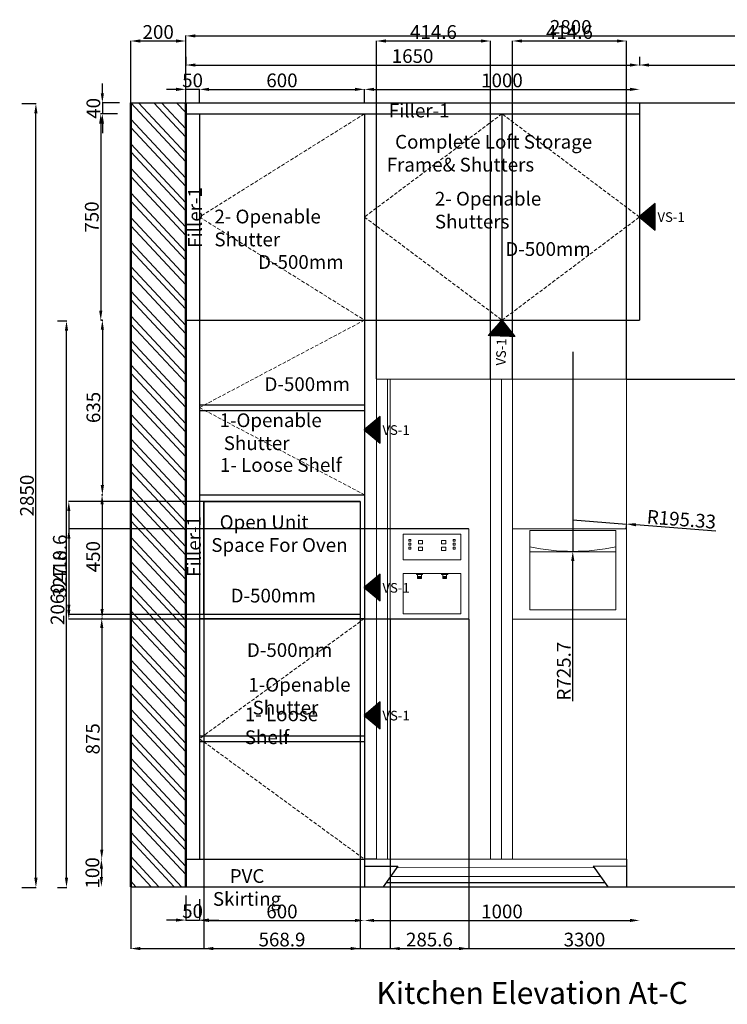
# Model space of a CAD drawing. Units: millimetres. Extents: x 407065 to 421840, y 1168257 to 1177792.
# Tile 1 of 17: x 407430 to 410003, y 1168257 to 1171838. Entities that reach past the tile are written whole.
import ezdxf

# ---------------------------------------------------------------- set-up
doc = ezdxf.new("R2010")
doc.units = ezdxf.units.MM
doc.linetypes.add('DASHED', pattern=[19.05, 12.7, -6.35])
for name, color, linetype, lineweight in [('A-ANNO-DIMS', 6, 'Continuous', 18), ('A-ANNO-TEXT', 30, 'Continuous', 18), ('A-EQPM', 8, 'Continuous', 18), ('A-FURN', 3, 'Continuous', 25), ('A-FURN-HIDN', 7, 'DASHED', 18), ('A-WALL', 7, 'Continuous', 50), ('A-WALL-PATT', 8, 'Continuous', 13)]:
    doc.layers.add(name, color=color, linetype=linetype, lineweight=lineweight)
doc.styles.get("Standard").update_dxf_attribs({"font": 'arial.ttf'})
doc.dimstyles.new('ISO-25', dxfattribs={"dimtxt": 50, "dimasz": 35, "dimexe": 1.25, "dimexo": 0.625, "dimtad": 1, "dimdec": 1, "dimtxsty": 'Standard', "dimcen": 35, "dimadec": 0, "dimazin": 0, "dimtfac": 1, "dimtdec": 1, "dimtmove": 0, "dimatfit": 3, "dimfxl": 1, "dimarcsym": 0})

# ---------------------------------------------------------------- blocks, each defined once
blk = doc.blocks.new('*D118')
at = {"layer": 'A-ANNO-DIMS', "color": 0, "lineweight": -2, "transparency": 16777216}
for p, q in [((407998.5, 1171584.4), (407963.5, 1171584.4)), ((408033.5, 1171554), (408033.5, 1171585.6)), ((408083.5, 1171584.4), (408033.5, 1171584.4)), ((408083.5, 1171541.4), (408083.5, 1171585.6)), ((408118.5, 1171584.4), (408153.5, 1171584.4))]:
    blk.add_line(p, q, dxfattribs=at)
at = {"layer": 'A-ANNO-DIMS', "color": 0, "transparency": 16777216}
for points in [[(407998.5, 1171590.2), (407998.5, 1171578.5), (408033.5, 1171584.4)], [(408118.5, 1171590.2), (408118.5, 1171578.5), (408083.5, 1171584.4)]]:
    blk.add_solid(points, dxfattribs=at)
at = {"layer": 'Defpoints', "color": 0, "transparency": 16777216}
for p in [(408033.5, 1171584.4), (408033.5, 1171553.4), (408083.5, 1171540.7)]:
    blk.add_point(p, dxfattribs=at)
at = {"layer": 'A-ANNO-DIMS', "color": 0, "transparency": 16777216, "insert": (408058.5, 1171610.5), "char_height": 50, "attachment_point": 5}
blk.add_mtext('50', dxfattribs=at)
blk = doc.blocks.new('*D119')
at = {"layer": 'A-ANNO-DIMS', "color": 0, "lineweight": -2, "transparency": 16777216}
for p, q in [((408083.5, 1171535.8), (408083.5, 1171585.6)), ((408118.5, 1171584.4), (408648.5, 1171584.4)), ((408683.5, 1171535.8), (408683.5, 1171585.6))]:
    blk.add_line(p, q, dxfattribs=at)
at = {"layer": 'A-ANNO-DIMS', "color": 0, "transparency": 16777216}
for points in [[(408118.5, 1171590.2), (408118.5, 1171578.5), (408083.5, 1171584.4)], [(408648.5, 1171590.2), (408648.5, 1171578.5), (408683.5, 1171584.4)]]:
    blk.add_solid(points, dxfattribs=at)
at = {"layer": 'Defpoints', "color": 0, "transparency": 16777216}
for p in [(408683.5, 1171584.4), (408083.5, 1171535.2), (408683.5, 1171535.2)]:
    blk.add_point(p, dxfattribs=at)
at = {"layer": 'A-ANNO-DIMS', "color": 0, "transparency": 16777216, "insert": (408383.5, 1171610.5), "char_height": 50, "attachment_point": 5}
blk.add_mtext('600', dxfattribs=at)
blk = doc.blocks.new('*D120')
at = {"layer": 'A-ANNO-DIMS', "color": 0, "lineweight": -2, "transparency": 16777216}
for p, q in [((408683.5, 1171585), (408683.5, 1171585.6)), ((408718.5, 1171584.4), (409648.5, 1171584.4)), ((409683.5, 1171585), (409683.5, 1171585.6))]:
    blk.add_line(p, q, dxfattribs=at)
at = {"layer": 'A-ANNO-DIMS', "color": 0, "transparency": 16777216}
for points in [[(408718.5, 1171590.2), (408718.5, 1171578.5), (408683.5, 1171584.4)], [(409648.5, 1171590.2), (409648.5, 1171578.5), (409683.5, 1171584.4)]]:
    blk.add_solid(points, dxfattribs=at)
at = {"layer": 'Defpoints', "color": 0, "transparency": 16777216}
for p in [(408683.5, 1171584.4), (409683.5, 1171584.4), (409683.5, 1171584.4)]:
    blk.add_point(p, dxfattribs=at)
at = {"layer": 'A-ANNO-DIMS', "color": 0, "transparency": 16777216, "insert": (409183.5, 1171610.5), "char_height": 50, "attachment_point": 5}
blk.add_mtext('1000', dxfattribs=at)
blk = doc.blocks.new('*D121')
at = {"layer": 'A-ANNO-DIMS', "color": 0, "lineweight": -2, "transparency": 16777216}
for p, q in [((408033.5, 1171702.7), (408033.5, 1171671.6)), ((409683.5, 1171702.7), (409683.5, 1171671.6)), ((408068.5, 1171672.8), (409648.5, 1171672.8))]:
    blk.add_line(p, q, dxfattribs=at)
at = {"layer": 'A-ANNO-DIMS', "color": 0, "transparency": 16777216}
for points in [[(408068.5, 1171678.6), (408068.5, 1171667), (408033.5, 1171672.8)], [(409648.5, 1171678.6), (409648.5, 1171667), (409683.5, 1171672.8)]]:
    blk.add_solid(points, dxfattribs=at)
at = {"layer": 'Defpoints', "color": 0, "transparency": 16777216}
for p in [(408033.5, 1171703.3), (409683.5, 1171703.3), (409683.5, 1171672.8)]:
    blk.add_point(p, dxfattribs=at)
at = {"layer": 'A-ANNO-DIMS', "color": 0, "transparency": 16777216, "insert": (408858.5, 1171699), "char_height": 50, "attachment_point": 5}
blk.add_mtext('1650', dxfattribs=at)
blk = doc.blocks.new('*D122')
at = {"layer": 'A-ANNO-DIMS', "color": 0, "lineweight": -2, "transparency": 16777216}
for p, q in [((409683.5, 1171673.4), (409683.5, 1171674.1)), ((409718.5, 1171672.8), (410798.5, 1171672.8)), ((410833.5, 1171673.4), (410833.5, 1171674.1))]:
    blk.add_line(p, q, dxfattribs=at)
at = {"layer": 'A-ANNO-DIMS', "color": 0, "transparency": 16777216}
for points in [[(409718.5, 1171678.6), (409718.5, 1171667), (409683.5, 1171672.8)], [(410798.5, 1171678.6), (410798.5, 1171667), (410833.5, 1171672.8)]]:
    blk.add_solid(points, dxfattribs=at)
at = {"layer": 'Defpoints', "color": 0, "transparency": 16777216}
for p in [(409683.5, 1171672.8), (410833.5, 1171672.8), (410833.5, 1171672.8)]:
    blk.add_point(p, dxfattribs=at)
at = {"layer": 'A-ANNO-DIMS', "color": 0, "transparency": 16777216, "insert": (410258.5, 1171699), "char_height": 50, "attachment_point": 5}
blk.add_mtext('1150', dxfattribs=at)
blk = doc.blocks.new('*D123')
at = {"layer": 'A-ANNO-DIMS', "color": 0, "lineweight": -2, "transparency": 16777216}
for p, q in [((408033.5, 1171744.1), (408033.5, 1171780)), ((408068.5, 1171778.7), (410798.5, 1171778.7)), ((410833.5, 1171744.1), (410833.5, 1171780))]:
    blk.add_line(p, q, dxfattribs=at)
at = {"layer": 'A-ANNO-DIMS', "color": 0, "transparency": 16777216}
for points in [[(408068.5, 1171784.5), (408068.5, 1171772.9), (408033.5, 1171778.7)], [(410798.5, 1171784.5), (410798.5, 1171772.9), (410833.5, 1171778.7)]]:
    blk.add_solid(points, dxfattribs=at)
at = {"layer": 'Defpoints', "color": 0, "transparency": 16777216}
for p in [(410833.5, 1171778.7), (408033.5, 1171743.5), (410833.5, 1171743.5)]:
    blk.add_point(p, dxfattribs=at)
at = {"layer": 'A-ANNO-DIMS', "color": 0, "transparency": 16777216, "insert": (409433.5, 1171804.9), "char_height": 50, "attachment_point": 5}
blk.add_mtext('2800', dxfattribs=at)
blk = doc.blocks.new('*D124')
at = {"layer": 'A-ANNO-DIMS', "color": 0, "lineweight": -2, "transparency": 16777216}
for p, q in [((407730.5, 1171570.2), (407730.5, 1171605.2)), ((407792.9, 1171535.2), (407729.2, 1171535.2)), ((407730.5, 1171535.2), (407730.5, 1171495.2)), ((407785.2, 1171495.2), (407729.2, 1171495.2)), ((407730.5, 1171460.2), (407730.5, 1171425.2))]:
    blk.add_line(p, q, dxfattribs=at)
at = {"layer": 'A-ANNO-DIMS', "color": 0, "transparency": 16777216}
for points in [[(407724.6, 1171570.2), (407736.3, 1171570.2), (407730.5, 1171535.2)], [(407724.6, 1171460.2), (407736.3, 1171460.2), (407730.5, 1171495.2)]]:
    blk.add_solid(points, dxfattribs=at)
at = {"layer": 'Defpoints', "color": 0, "transparency": 16777216}
for p in [(407793.6, 1171535.2), (407730.5, 1171495.2), (407785.8, 1171495.2)]:
    blk.add_point(p, dxfattribs=at)
at = {"layer": 'A-ANNO-DIMS', "color": 0, "transparency": 16777216, "insert": (407704.3, 1171515.2), "char_height": 50, "attachment_point": 5, "rotation": 90}
blk.add_mtext('40', dxfattribs=at)
blk = doc.blocks.new('*D125')
at = {"layer": 'A-ANNO-DIMS', "color": 0, "lineweight": -2, "transparency": 16777216}
for p, q in [((407729.8, 1171495.2), (407723.4, 1171495.2)), ((407724.6, 1171460.2), (407724.6, 1170780.2)), ((407729.8, 1170745.2), (407723.4, 1170745.2))]:
    blk.add_line(p, q, dxfattribs=at)
at = {"layer": 'A-ANNO-DIMS', "color": 0, "transparency": 16777216}
for points in [[(407718.8, 1171460.2), (407730.5, 1171460.2), (407724.6, 1171495.2)], [(407718.8, 1170780.2), (407730.5, 1170780.2), (407724.6, 1170745.2)]]:
    blk.add_solid(points, dxfattribs=at)
at = {"layer": 'Defpoints', "color": 0, "transparency": 16777216}
for p in [(407730.5, 1171495.2), (407724.6, 1170745.2), (407730.5, 1170745.2)]:
    blk.add_point(p, dxfattribs=at)
at = {"layer": 'A-ANNO-DIMS', "color": 0, "transparency": 16777216, "insert": (407698.5, 1171120.2), "char_height": 50, "attachment_point": 5, "rotation": 90}
blk.add_mtext('750', dxfattribs=at)
blk = doc.blocks.new('*D126')
at = {"layer": 'A-ANNO-DIMS', "color": 0, "lineweight": -2, "transparency": 16777216}
for p, q in [((407727.2, 1170745.2), (407731.7, 1170745.2)), ((407730.5, 1170710.2), (407730.5, 1170145.2)), ((407727.2, 1170110.2), (407731.7, 1170110.2))]:
    blk.add_line(p, q, dxfattribs=at)
at = {"layer": 'A-ANNO-DIMS', "color": 0, "transparency": 16777216}
for points in [[(407724.6, 1170710.2), (407736.3, 1170710.2), (407730.5, 1170745.2)], [(407724.6, 1170145.2), (407736.3, 1170145.2), (407730.5, 1170110.2)]]:
    blk.add_solid(points, dxfattribs=at)
at = {"layer": 'Defpoints', "color": 0, "transparency": 16777216}
for p in [(407726.6, 1170745.2), (407726.6, 1170110.2), (407730.5, 1170110.2)]:
    blk.add_point(p, dxfattribs=at)
at = {"layer": 'A-ANNO-DIMS', "color": 0, "transparency": 16777216, "insert": (407704.3, 1170427.7), "char_height": 50, "attachment_point": 5, "rotation": 90}
blk.add_mtext('635', dxfattribs=at)
blk = doc.blocks.new('*D127')
at = {"layer": 'A-ANNO-DIMS', "color": 0, "lineweight": -2, "transparency": 16777216}
for p, q in [((407731.1, 1170110.2), (407728.2, 1170110.2)), ((407729.5, 1170075.2), (407729.5, 1169695.2)), ((407731.1, 1169660.2), (407728.2, 1169660.2))]:
    blk.add_line(p, q, dxfattribs=at)
at = {"layer": 'A-ANNO-DIMS', "color": 0, "transparency": 16777216}
for points in [[(407723.6, 1170075.2), (407735.3, 1170075.2), (407729.5, 1170110.2)], [(407723.6, 1169695.2), (407735.3, 1169695.2), (407729.5, 1169660.2)]]:
    blk.add_solid(points, dxfattribs=at)
at = {"layer": 'Defpoints', "color": 0, "transparency": 16777216}
for p in [(407731.7, 1170110.2), (407729.5, 1169660.2), (407731.7, 1169660.2)]:
    blk.add_point(p, dxfattribs=at)
at = {"layer": 'A-ANNO-DIMS', "color": 0, "transparency": 16777216, "insert": (407703.3, 1169885.2), "char_height": 50, "attachment_point": 5, "rotation": 90}
blk.add_mtext('450', dxfattribs=at)
blk = doc.blocks.new('*D128')
at = {"layer": 'A-ANNO-DIMS', "color": 0, "lineweight": -2, "transparency": 16777216}
for p, q in [((407729, 1169660.2), (407727, 1169660.2)), ((407728.2, 1169625.2), (407728.2, 1168820.2)), ((407729, 1168785.2), (407727, 1168785.2))]:
    blk.add_line(p, q, dxfattribs=at)
at = {"layer": 'A-ANNO-DIMS', "color": 0, "transparency": 16777216}
for points in [[(407722.4, 1169625.2), (407734.1, 1169625.2), (407728.2, 1169660.2)], [(407722.4, 1168820.2), (407734.1, 1168820.2), (407728.2, 1168785.2)]]:
    blk.add_solid(points, dxfattribs=at)
at = {"layer": 'Defpoints', "color": 0, "transparency": 16777216}
for p in [(407729.7, 1169660.2), (407728.2, 1168785.2), (407729.7, 1168785.2)]:
    blk.add_point(p, dxfattribs=at)
at = {"layer": 'A-ANNO-DIMS', "color": 0, "transparency": 16777216, "insert": (407702.1, 1169222.7), "char_height": 50, "attachment_point": 5, "rotation": 90}
blk.add_mtext('875', dxfattribs=at)
blk = doc.blocks.new('*D129')
at = {"layer": 'A-ANNO-DIMS', "color": 0, "lineweight": -2, "transparency": 16777216}
for p, q in [((407726.3, 1168785.2), (407725.7, 1168785.2)), ((407727, 1168750.2), (407727, 1168720.2)), ((407726.3, 1168685.2), (407725.7, 1168685.2))]:
    blk.add_line(p, q, dxfattribs=at)
at = {"layer": 'A-ANNO-DIMS', "color": 0, "transparency": 16777216}
for points in [[(407721.1, 1168750.2), (407732.8, 1168750.2), (407727, 1168785.2)], [(407721.1, 1168720.2), (407732.8, 1168720.2), (407727, 1168685.2)]]:
    blk.add_solid(points, dxfattribs=at)
at = {"layer": 'Defpoints', "color": 0, "transparency": 16777216}
for p in [(407727, 1168785.2), (407727, 1168685.2), (407727, 1168685.2)]:
    blk.add_point(p, dxfattribs=at)
at = {"layer": 'A-ANNO-DIMS', "color": 0, "transparency": 16777216, "insert": (407700.8, 1168735.2), "char_height": 50, "attachment_point": 5, "rotation": 90}
blk.add_mtext('100', dxfattribs=at)
blk = doc.blocks.new('*D130')
at = {"layer": 'A-ANNO-DIMS', "color": 0, "lineweight": -2, "transparency": 16777216}
for p, q in [((407567.1, 1170742.4), (407601.3, 1170742.4)), ((407600.1, 1168717.4), (407600.1, 1170707.4)), ((407567.1, 1168682.4), (407601.3, 1168682.4))]:
    blk.add_line(p, q, dxfattribs=at)
at = {"layer": 'A-ANNO-DIMS', "color": 0, "transparency": 16777216}
for points in [[(407594.2, 1170707.4), (407605.9, 1170707.4), (407600.1, 1170742.4)], [(407594.2, 1168717.4), (407605.9, 1168717.4), (407600.1, 1168682.4)]]:
    blk.add_solid(points, dxfattribs=at)
at = {"layer": 'Defpoints', "color": 0, "transparency": 16777216}
for p in [(407566.4, 1170742.4), (407600.1, 1170742.4), (407566.4, 1168682.4)]:
    blk.add_point(p, dxfattribs=at)
at = {"layer": 'A-ANNO-DIMS', "color": 0, "transparency": 16777216, "insert": (407573.9, 1169712.4), "char_height": 50, "attachment_point": 5, "rotation": 90}
blk.add_mtext('2060', dxfattribs=at)
blk = doc.blocks.new('*D131')
at = {"layer": 'A-ANNO-DIMS', "color": 0, "lineweight": -2, "transparency": 16777216}
for p, q in [((407437.7, 1171532.4), (407490.1, 1171532.4)), ((407488.8, 1168717.4), (407488.8, 1171497.4)), ((407437.7, 1168682.4), (407490.1, 1168682.4))]:
    blk.add_line(p, q, dxfattribs=at)
at = {"layer": 'A-ANNO-DIMS', "color": 0, "transparency": 16777216}
for points in [[(407483, 1171497.4), (407494.7, 1171497.4), (407488.8, 1171532.4)], [(407483, 1168717.4), (407494.7, 1168717.4), (407488.8, 1168682.4)]]:
    blk.add_solid(points, dxfattribs=at)
at = {"layer": 'Defpoints', "color": 0, "transparency": 16777216}
for p in [(407437.1, 1171532.4), (407488.8, 1171532.4), (407437.1, 1168682.4)]:
    blk.add_point(p, dxfattribs=at)
at = {"layer": 'A-ANNO-DIMS', "color": 0, "transparency": 16777216, "insert": (407462.7, 1170107.4), "char_height": 50, "attachment_point": 5, "rotation": 90}
blk.add_mtext('2850', dxfattribs=at)
blk = doc.blocks.new('*D132')
at = {"layer": 'A-ANNO-DIMS', "color": 0, "lineweight": -2, "transparency": 16777216}
for p, q in [((408033.5, 1168653.1), (408033.5, 1168562.4)), ((408083.5, 1168639.9), (408083.5, 1168562.4)), ((407998.5, 1168563.7), (407963.5, 1168563.7)), ((408033.5, 1168563.7), (408083.5, 1168563.7)), ((408118.5, 1168563.7), (408153.5, 1168563.7))]:
    blk.add_line(p, q, dxfattribs=at)
at = {"layer": 'A-ANNO-DIMS', "color": 0, "transparency": 16777216}
for points in [[(407998.5, 1168569.5), (407998.5, 1168557.9), (408033.5, 1168563.7)], [(408118.5, 1168569.5), (408118.5, 1168557.9), (408083.5, 1168563.7)]]:
    blk.add_solid(points, dxfattribs=at)
at = {"layer": 'Defpoints', "color": 0, "transparency": 16777216}
for p in [(408033.5, 1168653.7), (408083.5, 1168640.5), (408083.5, 1168563.7)]:
    blk.add_point(p, dxfattribs=at)
at = {"layer": 'A-ANNO-DIMS', "color": 0, "transparency": 16777216, "insert": (408058.5, 1168589.9), "char_height": 50, "attachment_point": 5}
blk.add_mtext('50', dxfattribs=at)
blk = doc.blocks.new('*D133')
at = {"layer": 'A-ANNO-DIMS', "color": 0, "lineweight": -2, "transparency": 16777216}
for p, q in [((408083.5, 1168563.1), (408083.5, 1168563.7)), ((408118.5, 1168562.4), (408648.5, 1168562.4)), ((408683.5, 1168563.1), (408683.5, 1168563.7))]:
    blk.add_line(p, q, dxfattribs=at)
at = {"layer": 'A-ANNO-DIMS', "color": 0, "transparency": 16777216}
for points in [[(408118.5, 1168568.3), (408118.5, 1168556.6), (408083.5, 1168562.4)], [(408648.5, 1168568.3), (408648.5, 1168556.6), (408683.5, 1168562.4)]]:
    blk.add_solid(points, dxfattribs=at)
at = {"layer": 'Defpoints', "color": 0, "transparency": 16777216}
for p in [(408083.5, 1168562.4), (408683.5, 1168562.4), (408683.5, 1168562.4)]:
    blk.add_point(p, dxfattribs=at)
at = {"layer": 'A-ANNO-DIMS', "color": 0, "transparency": 16777216, "insert": (408383.5, 1168588.6), "char_height": 50, "attachment_point": 5}
blk.add_mtext('600', dxfattribs=at)
blk = doc.blocks.new('*D134')
at = {"layer": 'A-ANNO-DIMS', "color": 0, "lineweight": -2, "transparency": 16777216}
for p, q in [((408683.5, 1168563.1), (408683.5, 1168563.7)), ((408718.5, 1168562.4), (409648.5, 1168562.4)), ((409683.5, 1168563.1), (409683.5, 1168563.7))]:
    blk.add_line(p, q, dxfattribs=at)
at = {"layer": 'A-ANNO-DIMS', "color": 0, "transparency": 16777216}
for points in [[(408718.5, 1168568.3), (408718.5, 1168556.6), (408683.5, 1168562.4)], [(409648.5, 1168568.3), (409648.5, 1168556.6), (409683.5, 1168562.4)]]:
    blk.add_solid(points, dxfattribs=at)
at = {"layer": 'Defpoints', "color": 0, "transparency": 16777216}
for p in [(408683.5, 1168562.4), (409683.5, 1168562.4), (409683.5, 1168562.4)]:
    blk.add_point(p, dxfattribs=at)
at = {"layer": 'A-ANNO-DIMS', "color": 0, "transparency": 16777216, "insert": (409183.5, 1168588.6), "char_height": 50, "attachment_point": 5}
blk.add_mtext('1000', dxfattribs=at)
blk = doc.blocks.new('SHUTTER-HANDLE-MARK')
h = blk.add_hatch()
h.set_pattern_fill('ANSI32', color=256, scale=0.08)
h.set_pattern_definition([(45, (-3404.92366, -221.627), (-0.53881536726, 0.53881536726), []), (45, (-3404.56445, -221.627), (-0.53881536726, 0.53881536726), [])])
h.paths.add_polyline_path([(420059.2, 1176549.9), (420001.3, 1176501.2), (420059.2, 1176452.5)])
h = blk.add_hatch(color=256)
h.dxf.hatch_style = 1
h.paths.add_polyline_path([(420059.2, 1176549.9), (420001.3, 1176501.2), (420059.2, 1176452.5)])
blk = doc.blocks.new('*D208')
at = {"layer": 'A-ANNO-DIMS', "color": 0, "lineweight": -2, "transparency": 16777216}
for p, q in [((407833.5, 1168684.6), (407833.5, 1168458.9)), ((411133.5, 1168684.6), (411133.5, 1168458.9)), ((407868.5, 1168460.2), (411098.5, 1168460.2))]:
    blk.add_line(p, q, dxfattribs=at)
at = {"layer": 'A-ANNO-DIMS', "color": 0, "transparency": 16777216}
for points in [[(407868.5, 1168466), (407868.5, 1168454.4), (407833.5, 1168460.2)], [(411098.5, 1168466), (411098.5, 1168454.4), (411133.5, 1168460.2)]]:
    blk.add_solid(points, dxfattribs=at)
at = {"layer": 'Defpoints', "color": 0, "transparency": 16777216}
for p in [(407833.5, 1168685.2), (411133.5, 1168685.2), (411133.5, 1168460.2)]:
    blk.add_point(p, dxfattribs=at)
at = {"layer": 'A-ANNO-DIMS', "color": 0, "transparency": 16777216, "insert": (409483.5, 1168486.4), "char_height": 50, "attachment_point": 5}
blk.add_mtext('3300', dxfattribs=at)
blk = doc.blocks.new('*D209')
at = {"layer": 'A-ANNO-DIMS', "color": 0, "lineweight": -2, "transparency": 16777216}
for p, q in [((407833.5, 1171535.8), (407833.5, 1171761.4)), ((407868.5, 1171760.2), (407998.5, 1171760.2)), ((408033.5, 1171535.8), (408033.5, 1171761.4))]:
    blk.add_line(p, q, dxfattribs=at)
at = {"layer": 'A-ANNO-DIMS', "color": 0, "transparency": 16777216}
for points in [[(407868.5, 1171766), (407868.5, 1171754.4), (407833.5, 1171760.2)], [(407998.5, 1171766), (407998.5, 1171754.4), (408033.5, 1171760.2)]]:
    blk.add_solid(points, dxfattribs=at)
at = {"layer": 'Defpoints', "color": 0, "transparency": 16777216}
for p in [(408033.5, 1171760.2), (407833.5, 1171535.2), (408033.5, 1171535.2)]:
    blk.add_point(p, dxfattribs=at)
at = {"layer": 'A-ANNO-DIMS', "color": 0, "transparency": 16777216, "insert": (407933.5, 1171786.4), "char_height": 50, "attachment_point": 5}
blk.add_mtext('200', dxfattribs=at)
blk = doc.blocks.new('*D212')
at = {"layer": 'A-ANNO-DIMS', "color": 0, "lineweight": -2, "transparency": 16777216}
for p, q in [((409636.9, 1170530.8), (411359.8, 1170530.8)), ((411358.5, 1170495.8), (411358.5, 1168720.2)), ((409636.9, 1168685.2), (411359.8, 1168685.2))]:
    blk.add_line(p, q, dxfattribs=at)
at = {"layer": 'A-ANNO-DIMS', "color": 0, "transparency": 16777216}
for points in [[(411352.7, 1170495.8), (411364.4, 1170495.8), (411358.5, 1170530.8)], [(411352.7, 1168720.2), (411364.4, 1168720.2), (411358.5, 1168685.2)]]:
    blk.add_solid(points, dxfattribs=at)
at = {"layer": 'Defpoints', "color": 0, "transparency": 16777216}
for p in [(409636.3, 1170530.8), (409636.3, 1168685.2), (411358.5, 1168685.2)]:
    blk.add_point(p, dxfattribs=at)
at = {"layer": 'A-ANNO-DIMS', "color": 0, "transparency": 16777216, "insert": (411332.4, 1169608), "char_height": 50, "attachment_point": 5, "rotation": 90}
blk.add_mtext('1845.6', dxfattribs=at)
blk = doc.blocks.new('*D213')
at = {"layer": 'A-ANNO-DIMS', "color": 0, "lineweight": -2, "transparency": 16777216}
for p, q in [((408727, 1170531.4), (408727, 1171761.4)), ((408762, 1171760.2), (409106.7, 1171760.2)), ((409141.7, 1170531.4), (409141.7, 1171761.4))]:
    blk.add_line(p, q, dxfattribs=at)
at = {"layer": 'A-ANNO-DIMS', "color": 0, "transparency": 16777216}
for points in [[(408762, 1171766), (408762, 1171754.4), (408727, 1171760.2)], [(409106.7, 1171766), (409106.7, 1171754.4), (409141.7, 1171760.2)]]:
    blk.add_solid(points, dxfattribs=at)
at = {"layer": 'Defpoints', "color": 0, "transparency": 16777216}
for p in [(409141.7, 1171760.2), (408727, 1170530.8), (409141.7, 1170530.8)]:
    blk.add_point(p, dxfattribs=at)
at = {"layer": 'A-ANNO-DIMS', "color": 0, "transparency": 16777216, "insert": (408934.4, 1171786.4), "char_height": 50, "attachment_point": 5}
blk.add_mtext('414.6', dxfattribs=at)
blk = doc.blocks.new('*D214')
at = {"layer": 'A-ANNO-DIMS', "color": 0, "lineweight": -2, "transparency": 16777216}
for p, q in [((409221.7, 1170531.4), (409221.7, 1171761.4)), ((409256.7, 1171760.2), (409601.3, 1171760.2)), ((409636.3, 1170531.4), (409636.3, 1171761.4))]:
    blk.add_line(p, q, dxfattribs=at)
at = {"layer": 'A-ANNO-DIMS', "color": 0, "transparency": 16777216}
for points in [[(409256.7, 1171766), (409256.7, 1171754.4), (409221.7, 1171760.2)], [(409601.3, 1171766), (409601.3, 1171754.4), (409636.3, 1171760.2)]]:
    blk.add_solid(points, dxfattribs=at)
at = {"layer": 'Defpoints', "color": 0, "transparency": 16777216}
for p in [(409636.3, 1171760.2), (409221.7, 1170530.8), (409636.3, 1170530.8)]:
    blk.add_point(p, dxfattribs=at)
at = {"layer": 'A-ANNO-DIMS', "color": 0, "transparency": 16777216, "insert": (409429, 1171786.4), "char_height": 50, "attachment_point": 5}
blk.add_mtext('414.6', dxfattribs=at)
blk = doc.blocks.new('*D215')
at = {"layer": 'A-ANNO-DIMS', "color": 0, "lineweight": -2, "transparency": 16777216}
for p, q in [((408777, 1169657.4), (408777, 1168458.9)), ((409062.6, 1169657.4), (409062.6, 1168458.9)), ((408812, 1168460.2), (409027.6, 1168460.2))]:
    blk.add_line(p, q, dxfattribs=at)
at = {"layer": 'A-ANNO-DIMS', "color": 0, "transparency": 16777216}
for points in [[(408812, 1168466), (408812, 1168454.4), (408777, 1168460.2)], [(409027.6, 1168466), (409027.6, 1168454.4), (409062.6, 1168460.2)]]:
    blk.add_solid(points, dxfattribs=at)
at = {"layer": 'Defpoints', "color": 0, "transparency": 16777216}
for p in [(408777, 1169658), (409062.6, 1169658), (409062.6, 1168460.2)]:
    blk.add_point(p, dxfattribs=at)
at = {"layer": 'A-ANNO-DIMS', "color": 0, "transparency": 16777216, "insert": (408919.8, 1168486.4), "char_height": 50, "attachment_point": 5}
blk.add_mtext('285.6', dxfattribs=at)
blk = doc.blocks.new('*D216')
at = {"layer": 'A-ANNO-DIMS', "color": 0, "lineweight": -2, "transparency": 16777216}
for p, q in [((409062, 1169985.8), (407607.3, 1169985.8)), ((407608.5, 1169950.8), (407608.5, 1169693)), ((409062, 1169658), (407607.3, 1169658))]:
    blk.add_line(p, q, dxfattribs=at)
at = {"layer": 'A-ANNO-DIMS', "color": 0, "transparency": 16777216}
for points in [[(407602.7, 1169950.8), (407614.4, 1169950.8), (407608.5, 1169985.8)], [(407602.7, 1169693), (407614.4, 1169693), (407608.5, 1169658)]]:
    blk.add_solid(points, dxfattribs=at)
at = {"layer": 'Defpoints', "color": 0, "transparency": 16777216}
for p in [(409062.6, 1169985.8), (407608.5, 1169658), (409062.6, 1169658)]:
    blk.add_point(p, dxfattribs=at)
at = {"layer": 'A-ANNO-DIMS', "color": 0, "transparency": 16777216, "insert": (407582.4, 1169821.9), "char_height": 50, "attachment_point": 5, "rotation": 90}
blk.add_mtext('327.8', dxfattribs=at)
blk = doc.blocks.new('*D217')
at = {"layer": 'A-ANNO-DIMS', "color": 0, "lineweight": -2, "transparency": 16777216}
for p, q in [((408099.1, 1170085.1), (408099.1, 1168458.9)), ((408668, 1170085.1), (408668, 1168458.9)), ((408134.1, 1168460.2), (408633, 1168460.2))]:
    blk.add_line(p, q, dxfattribs=at)
at = {"layer": 'A-ANNO-DIMS', "color": 0, "transparency": 16777216}
for points in [[(408134.1, 1168466), (408134.1, 1168454.4), (408099.1, 1168460.2)], [(408633, 1168466), (408633, 1168454.4), (408668, 1168460.2)]]:
    blk.add_solid(points, dxfattribs=at)
at = {"layer": 'Defpoints', "color": 0, "transparency": 16777216}
for p in [(408099.1, 1170085.7), (408668, 1170085.7), (408668, 1168460.2)]:
    blk.add_point(p, dxfattribs=at)
at = {"layer": 'A-ANNO-DIMS', "color": 0, "transparency": 16777216, "insert": (408383.6, 1168486.4), "char_height": 50, "attachment_point": 5}
blk.add_mtext('568.9', dxfattribs=at)
blk = doc.blocks.new('*D218')
at = {"layer": 'A-ANNO-DIMS', "color": 0, "lineweight": -2, "transparency": 16777216}
for p, q in [((408667.4, 1170085.7), (407607.3, 1170085.7)), ((407608.5, 1170050.7), (407608.5, 1169710.1)), ((408667.4, 1169675.1), (407607.3, 1169675.1))]:
    blk.add_line(p, q, dxfattribs=at)
at = {"layer": 'A-ANNO-DIMS', "color": 0, "transparency": 16777216}
for points in [[(407602.7, 1170050.7), (407614.4, 1170050.7), (407608.5, 1170085.7)], [(407602.7, 1169710.1), (407614.4, 1169710.1), (407608.5, 1169675.1)]]:
    blk.add_solid(points, dxfattribs=at)
at = {"layer": 'Defpoints', "color": 0, "transparency": 16777216}
for p in [(408668, 1170085.7), (407608.5, 1169675.1), (408668, 1169675.1)]:
    blk.add_point(p, dxfattribs=at)
at = {"layer": 'A-ANNO-DIMS', "color": 0, "transparency": 16777216, "insert": (407582.4, 1169880.4), "char_height": 50, "attachment_point": 5, "rotation": 90}
blk.add_mtext('410.6', dxfattribs=at)
blk = doc.blocks.new('*D240')
at = {"layer": 'A-ANNO-DIMS', "color": 0, "lineweight": -2, "transparency": 16777216}
for p, q in [((409441, 1170630), (409441, 1169904.3)), ((409441, 1169360), (409441, 1169869.3))]:
    blk.add_line(p, q, dxfattribs=at)
at = {"layer": 'A-ANNO-DIMS', "color": 0, "transparency": 16777216}
blk.add_solid([(409435.2, 1169869.3), (409446.8, 1169869.3), (409441, 1169904.3)], dxfattribs=at)
at = {"layer": 'Defpoints', "color": 0, "transparency": 16777216}
for p in [(409441, 1170630), (409441, 1169904.3)]:
    blk.add_point(p, dxfattribs=at)
at = {"layer": 'A-ANNO-DIMS', "color": 0, "transparency": 16777216, "insert": (409414.8, 1169468.9), "char_height": 50, "attachment_point": 5, "rotation": 89.9962}
blk.add_mtext('R725.7', dxfattribs=at)
blk = doc.blocks.new('*D241')
at = {"layer": 'A-ANNO-DIMS', "color": 0, "lineweight": -2, "transparency": 16777216}
for p, q in [((409441, 1170019.2), (409635.8, 1170003.9)), ((409961.5, 1169978.4), (409670.7, 1170001.2))]:
    blk.add_line(p, q, dxfattribs=at)
at = {"layer": 'A-ANNO-DIMS', "color": 0, "transparency": 16777216}
blk.add_solid([(409671.1, 1170007), (409670.2, 1169995.4), (409635.8, 1170003.9)], dxfattribs=at)
at = {"layer": 'Defpoints', "color": 0, "transparency": 16777216}
for p in [(409441, 1170019.2), (409635.8, 1170003.9)]:
    blk.add_point(p, dxfattribs=at)
at = {"layer": 'A-ANNO-DIMS', "color": 0, "transparency": 16777216, "insert": (409835.6, 1170014.6), "char_height": 50, "attachment_point": 5, "rotation": 355.5239}
blk.add_mtext('R195.33', dxfattribs=at)

msp = doc.modelspace()

# ---------------------------------------------------------------- hatches: boundary and pattern name
at = {"layer": 'A-WALL-PATT'}
h = msp.add_hatch(dxfattribs=at)
h.set_pattern_fill('ANSI32', color=256, scale=6.4, angle=88)
h.set_pattern_definition([(133, (-5768.25, -464.17), (-44.5833217, -41.57462), []), (133, (-5767.245, -435.45), (-44.5833217, -41.57462), [])])
h.paths.add_polyline_path([(408033.5433, 1171535.1988), (407833.5433, 1171535.1988), (407833.5433, 1168685.1988), (408033.5433, 1168685.1988)])

# ---------------------------------------------------------------- linework, layer by layer
at = {"layer": 'A-EQPM'}
for p, q in [((408727.047, 1168785.1988), (408727.047, 1170530.7673)), ((408727.047, 1170530.7673), (409636.3246, 1170530.7673)), ((408767.047, 1168785.1988), (408767.047, 1170530.7673)), ((408777.047, 1168785.1988), (408777.047, 1170530.7673)), ((409141.6858, 1170530.7673), (409141.6858, 1168785.1988)), ((409181.6858, 1170530.7673), (409181.6858, 1168785.1988)), ((409221.6858, 1170530.7673), (409221.6858, 1168785.1988)), ((409636.3246, 1170530.7673), (409636.3246, 1168785.1988)), ((409221.6858, 1169985.79), (409636.3246, 1169985.79)), ((409284.331, 1169902.5962), (409597.7663, 1169902.5962)), ((408876.501, 1169812.8191), (408890.575, 1169812.8191)), ((408876.501, 1169812.3613), (408890.575, 1169812.3613)), ((408876.501, 1169810.4478), (408890.575, 1169810.4478)), ((408876.501, 1169809.9624), (408890.575, 1169809.9624)), ((408876.501, 1169806.6731), (408890.575, 1169806.6731)), ((408982.0023, 1169812.8191), (408967.9283, 1169812.8191)), ((408982.0023, 1169812.3613), (408967.9283, 1169812.3613)), ((408982.0023, 1169810.4478), (408967.9283, 1169810.4478)), ((408982.0023, 1169809.9624), (408967.9283, 1169809.9624)), ((408982.0023, 1169806.6731), (408967.9283, 1169806.6731)), ((409221.6858, 1169657.9831), (409636.3246, 1169657.9831)), ((408727.047, 1168785.1988), (409636.3246, 1168785.1988)), ((408801.5867, 1168755.1904), (409519.7246, 1168753.1834)), ((409636.3246, 1168760.0712), (409514.7707, 1168760.0712)), ((408778.1721, 1168722.635), (409541.6958, 1168722.635))]:
    msp.add_line(p, q, dxfattribs=at)
for points in [[(408777.047, 1169657.9831), (409062.6226, 1169657.9831), (409062.6226, 1169985.79), (408777.047, 1169985.79)], [(409284.331, 1169979.8023), (409597.7663, 1169979.8023), (409597.7663, 1169691.8132), (409284.331, 1169691.8132)], [(409034.4605, 1169966.6384), (408824.0428, 1169966.6384), (408824.0428, 1169873.2129), (409034.4605, 1169873.2129)], [(408845.4354, 1169947.8495), (408852.048, 1169947.8495), (408852.048, 1169940.9553), (408845.4354, 1169940.9553)], [(408879.6544, 1169944.1523), (408894.3169, 1169944.1523), (408894.3169, 1169931.8001), (408879.6544, 1169931.8001)], [(408978.8489, 1169944.1523), (408964.1864, 1169944.1523), (408964.1864, 1169931.8001), (408978.8489, 1169931.8001)], [(409013.0679, 1169947.8495), (409006.4554, 1169947.8495), (409006.4554, 1169940.9553), (409013.0679, 1169940.9553)], [(408845.4354, 1169934.061), (408852.048, 1169934.061), (408852.048, 1169927.1668), (408845.4354, 1169927.1668)], [(408845.4354, 1169919.698), (408852.048, 1169919.698), (408852.048, 1169912.8037), (408845.4354, 1169912.8037)], [(408879.6544, 1169920.0224), (408894.3169, 1169920.0224), (408894.3169, 1169907.6702), (408879.6544, 1169907.6702)], [(408978.8489, 1169920.0224), (408964.1864, 1169920.0224), (408964.1864, 1169907.6702), (408978.8489, 1169907.6702)], [(409013.0679, 1169934.061), (409006.4554, 1169934.061), (409006.4554, 1169927.1668), (409013.0679, 1169927.1668)], [(409013.0679, 1169919.698), (409006.4554, 1169919.698), (409006.4554, 1169912.8037), (409013.0679, 1169912.8037)], [(409034.4605, 1169677.1346), (408824.0428, 1169677.1346), (408824.0428, 1169824.2678), (409034.4605, 1169824.2678)], [(408872.3552, 1169824.2678), (408894.6288, 1169824.2678), (408894.6288, 1169822.0238), (408872.3552, 1169822.0238)], [(408872.3552, 1169822.0238), (408894.6288, 1169822.0238), (408894.6288, 1169819.7798), (408872.3552, 1169819.7798)], [(408876.501, 1169819.7798), (408890.575, 1169819.7798), (408890.575, 1169805.8584), (408876.501, 1169805.8584)], [(408986.1481, 1169824.2678), (408963.8746, 1169824.2678), (408963.8746, 1169822.0238), (408986.1481, 1169822.0238)], [(408986.1481, 1169822.0238), (408963.8746, 1169822.0238), (408963.8746, 1169819.7798), (408986.1481, 1169819.7798)], [(408982.0023, 1169819.7798), (408967.9283, 1169819.7798), (408967.9283, 1169805.8584), (408982.0023, 1169805.8584)]]:
    msp.add_lwpolyline(points, close=True, dxfattribs=at)
for centre, radius, start, end in [((409441.0486, 1170019.1828), 195.3275, 350.1564704, 1.316737), ((409441.0486, 1170629.9782), 725.6939, 257.528407, 282.471593)]:
    msp.add_arc(centre, radius, start, end, dxfattribs=at)
at = {"layer": 'A-FURN'}
for p, q in [((407833.5433, 1171535.1988), (411133.5433, 1171535.1988)), ((409683.5433, 1171535.1988), (409683.5433, 1170745.1988)), ((408033.5433, 1171495.1988), (409683.5433, 1171495.1988)), ((408083.5433, 1171495.1988), (408083.5433, 1168785.1988)), ((408683.5433, 1171495.1988), (408683.5433, 1168685.1988)), ((409183.5433, 1171495.1988), (409183.5433, 1170745.1988)), ((408033.5433, 1170745.1988), (409683.5433, 1170745.1988)), ((408083.5433, 1170437.1988), (408683.5433, 1170437.1988)), ((408083.5433, 1170417.1988), (408683.5433, 1170417.1988)), ((408083.5433, 1170110.1988), (408683.5433, 1170110.1988)), ((408083.5433, 1169660.1988), (408683.5433, 1169660.1988)), ((408083.5433, 1169233.1988), (408683.5433, 1169233.1988)), ((408083.5433, 1169213.1988), (408683.5433, 1169213.1988)), ((408033.5433, 1168785.1988), (408683.5433, 1168785.1988)), ((408727.047, 1168785.1988), (408683.5433, 1168785.1988)), ((409636.3246, 1168785.1988), (409636.3246, 1168685.1988)), ((408683.5433, 1168760.0712), (408805.0972, 1168760.0712)), ((408805.0972, 1168760.0712), (408751.2471, 1168685.1988)), ((409514.7707, 1168760.0712), (409568.6208, 1168685.1988)), ((408762.5591, 1168700.9268), (409558.0576, 1168699.8858)), ((407833.5433, 1168685.1988), (411133.5433, 1168685.1988)), ((408683.5433, 1168685.1988), (408751.2471, 1168685.1988)), ((409568.6208, 1168685.1988), (409636.3246, 1168685.1988))]:
    msp.add_line(p, q, dxfattribs=at)
for points in [[(409740.51, 1171169.6864), (409682.5869, 1171121.0026), (409740.51, 1171072.3188)], [(409132.8726, 1170689.0057), (409183.5433, 1170745.1988), (409230.1812, 1170685.6161)], [(408740.51, 1170395.2865), (408682.5869, 1170346.6027), (408740.51, 1170297.9189)], [(408099.149, 1170085.7275), (408668.025, 1170085.7275), (408668.025, 1169675.0929), (408099.149, 1169675.0929)], [(408740.51, 1169821.3848), (408682.5869, 1169772.701), (408740.51, 1169724.0172)], [(408740.51, 1169356.862), (408682.5869, 1169308.1782), (408740.51, 1169259.4944)]]:
    msp.add_lwpolyline(points, close=True, dxfattribs=at)
at = {"layer": 'A-FURN-HIDN'}
for p, q in [((408683.5433, 1171495.1988), (408083.5433, 1171120.1988)), ((409183.5433, 1171495.1988), (408683.5433, 1171120.1988)), ((409683.5433, 1171120.1988), (409183.5433, 1171495.1988)), ((408083.5433, 1171120.1988), (408683.5433, 1170745.1988)), ((408683.5433, 1171120.1988), (409183.5433, 1170745.1988)), ((409183.5433, 1170745.1988), (409683.5433, 1171120.1988)), ((408683.5433, 1170745.1988), (408083.5433, 1170427.1988)), ((408083.5433, 1170427.1988), (408683.5433, 1170110.1988)), ((408683.5433, 1169660.1988), (408083.5433, 1169223.1988)), ((408083.5433, 1169223.1988), (408683.5433, 1168785.1988))]:
    msp.add_line(p, q, dxfattribs=at)
at = {"layer": 'A-WALL'}
for p, q in [((407833.5433, 1171535.1988), (407833.5433, 1168685.1988)), ((408033.5433, 1171535.1988), (408033.5433, 1168685.1988))]:
    msp.add_line(p, q, dxfattribs=at)

# ---------------------------------------------------------------- block references
at = {"layer": 'A-FURN'}
for p in [(-10318.6901, -5380.1656), (-11318.6901, -6154.5655), (-11318.6901, -6728.4672), (-11318.6901, -7192.99)]:
    msp.add_blockref('SHUTTER-HANDLE-MARK', p, dxfattribs=at)
at = {"layer": 'A-FURN', "extrusion": (0, 0, -1), "zscale": -1, "rotation": 271.994985739721}
msp.add_blockref('SHUTTER-HANDLE-MARK', (-1599592.7066, 1549535.5043), dxfattribs=at)

# ---------------------------------------------------------------- texts
at = {"layer": 'A-ANNO-TEXT', "attachment_point": 1}
for s, width, insert, char_height in [('     Filler-1', 382.409863, (408695.5483, 1171532.3295), 50), ('  Complete Loft Storage     Frame& Shutters', 910.917662, (408764.3436, 1171418.7829), 50), ('2- Openable Shutters', 467.834353, (408939.5491, 1171211.7808), 50), ('2- Openable Shutter', 467.834353, (408137.897, 1171146.9435), 50), ('VS-1', 382.409863, (409748.973, 1171137.5022), 35), ('  D-500mm', 382.409863, (409165.29, 1171028.7674), 50), ('  D-500mm', 382.409863, (408266.3298, 1170981.6462), 50), ('  D-500mm', 382.409863, (408289.5514, 1170537.3753), 50), ('     1-Openable\\P      Shutter', 520.083559, (408080.2453, 1170406.197), 50), ('VS-1', 382.409863, (408748.973, 1170363.1022), 35), ('1- Loose Shelf', 464.175444, (408158.0859, 1170243.5987), 50), ('  Open Unit\\PSpace For Oven', 517.500852, (408126.5507, 1170035.9209), 50), ('  D-500mm', 382.409863, (408166.3724, 1169768.5558), 50), ('VS-1', 382.409863, (408748.973, 1169789.2006), 35), ('  D-500mm', 382.409863, (408225.6064, 1169570.4892), 50), ('     1-Openable\\P      Shutter', 520.083559, (408184.9778, 1169444.4339), 50), ('1- Loose Shelf', 382.409863, (408248.5983, 1169336.8923), 50), ('VS-1', 382.409863, (408748.973, 1169324.6778), 35), ('    PVC Skirting', 382.409863, (408132.4523, 1168748.9501), 50), ('Kitchen Elevation At-C', 1357.183536, (408726.8878, 1168338.8718), 80)]:
    msp.add_mtext_dynamic_manual_height_columns(s, width=width, gutter_width=12.5, heights=[0], dxfattribs=dict(at, insert=insert, char_height=char_height))
at = {"layer": 'A-ANNO-TEXT'}
for s, insert, char_height, attachment_point, rotation in [('     Filler-1', (408042.3906, 1170931.5456), 50, 1, 90), ('VS-1', (409164.7427, 1170679.4273), 35, 3, 88.0050143), ('     Filler-1', (408038.2228, 1169735.3101), 50, 1, 90)]:
    msp.add_mtext_dynamic_manual_height_columns(s, width=382.409863, gutter_width=12.5, heights=[0], dxfattribs=dict(at, insert=insert, char_height=char_height, attachment_point=attachment_point, rotation=rotation))

# ---------------------------------------------------------------- dimensions: what is measured, and where the dimension line sits
at = {"layer": 'A-ANNO-DIMS'}
for base, p1, p2, override, picture, middle in [((408033.5433, 1171760.1988), (407833.5433, 1171535.1988), (408033.5433, 1171535.1988), {"dimdec": 0, "dimlfac": 1, "dimrnd": 0, "dimzin": 0, "dimdsep": 46, "dimlunit": 2}, '*D209', (407933.5433, 1171786.3524)), ((410833.5433, 1171778.705), (408033.5433, 1171743.4929), (410833.5433, 1171743.4929), {"dimclrd": 0, "dimclre": 0, "dimclrt": 0}, '*D123', (409433.5433, 1171804.8586)), ((409141.6858, 1171760.1988), (408727.047, 1170530.7673), (409141.6858, 1170530.7673), {"dimdec": 1, "dimlfac": 1, "dimrnd": 0, "dimzin": 0, "dimdsep": 46, "dimlunit": 2}, '*D213', (408934.3664, 1171786.3524)), ((409636.3246, 1171760.1988), (409221.6858, 1170530.7673), (409636.3246, 1170530.7673), {"dimdec": 1, "dimlfac": 1, "dimrnd": 0, "dimzin": 0, "dimdsep": 46, "dimlunit": 2}, '*D214', (409429.0052, 1171786.3524)), ((409683.5433, 1171672.8068), (408033.5433, 1171703.2931), (409683.5433, 1171703.2931), {"dimclrd": 0, "dimclre": 0, "dimclrt": 0}, '*D121', (408858.5433, 1171698.9605)), ((410833.5433, 1171672.8068), (409683.5433, 1171672.8068), (410833.5433, 1171672.8068), {"dimclrd": 0, "dimclre": 0, "dimclrt": 0}, '*D122', (410258.5433, 1171698.9605)), ((408683.5433, 1171584.3788), (408083.5433, 1171535.1988), (408683.5433, 1171535.1988), {"dimclrd": 0, "dimclre": 0, "dimclrt": 0}, '*D119', (408383.5433, 1171610.5324)), ((409683.5433, 1171584.3788), (408683.5433, 1171584.3788), (409683.5433, 1171584.3788), {"dimclrd": 0, "dimclre": 0, "dimclrt": 0}, '*D120', (409183.5433, 1171610.5324)), ((408668.025, 1168460.1988), (408099.149, 1170085.7275), (408668.025, 1170085.7275), {"dimdec": 1, "dimlfac": 1, "dimrnd": 0, "dimzin": 0, "dimdsep": 46, "dimlunit": 2}, '*D217', (408383.587, 1168486.3524)), ((409062.6226, 1168460.1988), (408777.047, 1169657.9831), (409062.6226, 1169657.9831), {"dimdec": 1, "dimlfac": 1, "dimrnd": 0, "dimzin": 0, "dimdsep": 46, "dimlunit": 2}, '*D215', (408919.8348, 1168486.3524)), ((411133.5433, 1168460.1988), (407833.5433, 1168685.1988), (411133.5433, 1168685.1988), {"dimdec": 0, "dimlfac": 1, "dimrnd": 0, "dimzin": 0, "dimdsep": 46, "dimlunit": 2}, '*D208', (409483.5433, 1168486.3695)), ((408683.5433, 1168562.4464), (408083.5433, 1168562.4464), (408683.5433, 1168562.4464), {"dimclrd": 0, "dimclre": 0, "dimclrt": 0}, '*D133', (408383.5433, 1168588.6)), ((409683.5433, 1168562.4464), (408683.5433, 1168562.4464), (409683.5433, 1168562.4464), {"dimclrd": 0, "dimclre": 0, "dimclrt": 0}, '*D134', (409183.5433, 1168588.6))]:
    dim = msp.add_linear_dim(base=base, p1=p1, p2=p2, dimstyle='ISO-25', override=override, dxfattribs=at)
    dim.commit()
    dim.dimension.update_dxf_attribs({"geometry": picture, "text_midpoint": middle})
for base, p1, p2, picture, middle in [((408033.5433, 1171584.3788), (408083.5433, 1171540.7263), (408033.5433, 1171553.3771), '*D118', (408058.5433, 1171584.3788)), ((408083.5433, 1168563.6964), (408033.5433, 1168653.7363), (408083.5433, 1168640.5417), '*D132', (408058.5433, 1168563.6964))]:
    dim = msp.add_linear_dim(base=base, p1=p1, p2=p2, dimstyle='ISO-25', override={"dimclrd": 0, "dimclre": 0, "dimclrt": 0}, dxfattribs=at)
    dim.commit()
    dim.dimension.update_dxf_attribs({"geometry": picture, "text_midpoint": middle, "dimtype": 160})
for base, p1, p2, picture, middle in [((407730.4586, 1171495.1988), (407793.5533, 1171535.1988), (407785.7877, 1171495.1988), '*D124', (407730.4586, 1171515.1988)), ((407726.969, 1168685.1988), (407726.969, 1168785.1988), (407726.969, 1168685.1988), '*D129', (407726.969, 1168735.1988))]:
    dim = msp.add_linear_dim(base=base, p1=p1, p2=p2, angle=90, dimstyle='ISO-25', override={"dimclrd": 0, "dimclre": 0, "dimclrt": 0}, dxfattribs=at)
    dim.commit()
    dim.dimension.update_dxf_attribs({"geometry": picture, "text_midpoint": middle, "dimtype": 160})
for base, p1, p2, override, picture, middle in [((407488.8402, 1171532.4021), (407437.1126, 1168682.4021), (407437.1126, 1171532.4021), {"dimclrd": 0, "dimclre": 0, "dimclrt": 0}, '*D131', (407462.6866, 1170107.4021)), ((407724.6252, 1170745.1988), (407730.4586, 1171495.1988), (407730.4586, 1170745.1988), {"dimclrd": 0, "dimclre": 0, "dimclrt": 0}, '*D125', (407698.4716, 1171120.1988)), ((407600.0546, 1170742.4021), (407566.4317, 1168682.4021), (407566.4317, 1170742.4021), {"dimclrd": 0, "dimclre": 0, "dimclrt": 0}, '*D130', (407573.9009, 1169712.4021)), ((407730.4586, 1170110.1988), (407726.6044, 1170745.1988), (407726.6044, 1170110.1988), {"dimclrd": 0, "dimclre": 0, "dimclrt": 0}, '*D126', (407704.2879, 1170427.6988)), ((411358.5433, 1168685.1988), (409636.3246, 1170530.7673), (409636.3246, 1168685.1988), {"dimdec": 1, "dimlfac": 1, "dimrnd": 0, "dimzin": 0, "dimdsep": 46, "dimlunit": 2}, '*D212', (411332.3896, 1169607.9831)), ((407729.469, 1169660.1988), (407731.7086, 1170110.1988), (407731.7086, 1169660.1988), {"dimclrd": 0, "dimclre": 0, "dimclrt": 0}, '*D127', (407703.3153, 1169885.1988)), ((407608.5433, 1169675.0929), (408668.025, 1170085.7275), (408668.025, 1169675.0929), {"dimdec": 1, "dimlfac": 1, "dimrnd": 0, "dimzin": 0, "dimdsep": 46, "dimlunit": 2}, '*D218', (407582.3896, 1169880.4102)), ((407608.5433, 1169657.9831), (409062.6226, 1169985.79), (409062.6226, 1169657.9831), {"dimdec": 1, "dimlfac": 1, "dimrnd": 0, "dimzin": 0, "dimdsep": 46, "dimlunit": 2}, '*D216', (407582.3726, 1169821.8865)), ((407728.219, 1168785.1988), (407729.6513, 1169660.1988), (407729.6513, 1168785.1988), {"dimclrd": 0, "dimclre": 0, "dimclrt": 0}, '*D128', (407702.0653, 1169222.6988))]:
    dim = msp.add_linear_dim(base=base, p1=p1, p2=p2, angle=90, dimstyle='ISO-25', override=override, dxfattribs=at)
    dim.commit()
    dim.dimension.update_dxf_attribs({"geometry": picture, "text_midpoint": middle})
dim = msp.add_radius_dim(center=(409441.0486, 1170629.9782), mpoint=(409441, 1169904.2843), dimstyle='ISO-25', override={"dimdec": 1, "dimlfac": 1, "dimrnd": 0, "dimzin": 0, "dimdsep": 46, "dimlunit": 2}, dxfattribs=at)
dim.commit()
dim.dimension.update_dxf_attribs({"geometry": '*D240', "text_midpoint": (409440.9708, 1169468.8679), "dimtype": 164})
dim = msp.add_radius_dim(center=(409441.0486, 1170019.1828), mpoint=(409635.7804, 1170003.9389), dimstyle='ISO-25', override={"dimdec": 2, "dimlfac": 1, "dimrnd": 0, "dimzin": 0, "dimdsep": 46, "dimlunit": 2}, dxfattribs=at)
dim.commit()
dim.dimension.update_dxf_attribs({"geometry": '*D241', "text_midpoint": (409835.5544, 1170014.5511)})

doc.saveas('drawing.dxf')
